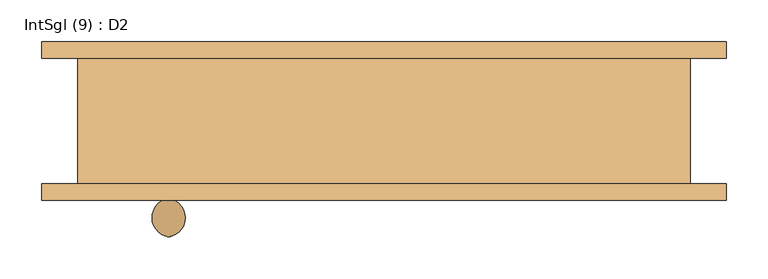
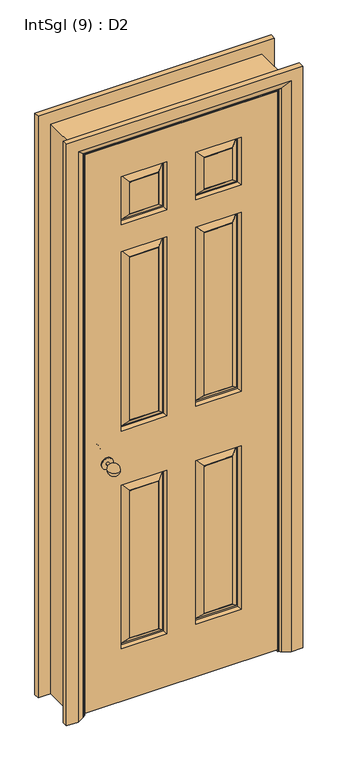
"""IFC4 building model written with IfcOpenShell, lengths in millimetres: door geometry, IntSgl (9) : D2."""

from ifc_helpers import new_model, si_unit, point, frame, origin, place, context, project, spatial, polyline, circle_curve, ellipse_curve, trimmed, outline, extrude, faceted_brep, source, transform, mapped, element, save
from ifc_brep_helpers import plane_surface, cylinder_surface, revolved_surface, advanced_brep


def intsgl_9_d2_a593ccd7(model_context):
    return source(origin(), model_context, "Body", "SolidModel", [
        advanced_brep(
        [(-253.0, -18.0, 900.0), (-263.0, -18.0, 900.0), (-258.0, 26.437411, 900.0), (-253.0, -33.0, 900.0), (-263.0, -33.0, 900.0), (-278.0, -37.0, 900.0), (-238.0, -37.0, 900.0), (-278.0, -33.0, 900.0), (-238.0, -33.0, 900.0)],
        [
            (0, 1, circle_curve(frame((-258.0, -18.0, 900.0), z_axis=(0.0, 1.0, 0.0), x_axis=(-1.0, 0.0, 0.0)), 5.0)),
            (1, 2, circle_curve(frame((-254.8115138, 3.5786495, 900.0), z_axis=(0.0, 0.0, -1.0), x_axis=(0.0, -1.0, 0.0)), 23.0800654)),
            (2, 0, circle_curve(frame((-261.1884862, 3.5786495, 900.0), z_axis=(0.0, 0.0, -1.0), x_axis=(0.0, -1.0, 0.0)), 23.0800654)),
            (1, 0, circle_curve(frame((-258.0, -18.0, 900.0), z_axis=(0.0, 1.0, 0.0), x_axis=(-1.0, 0.0, 0.0)), 5.0)),
            (0, 3),
            (3, 4, circle_curve(frame((-258.0, -33.0, 900.0), z_axis=(0.0, 1.0, 0.0), x_axis=(-1.0, 0.0, 0.0)), 5.0)),
            (4, 1),
            (4, 3, circle_curve(frame((-258.0, -33.0, 900.0), z_axis=(0.0, 1.0, 0.0), x_axis=(-1.0, 0.0, 0.0)), 5.0)),
            (5, 6, circle_curve(frame((-258.0, -37.0, 900.0), z_axis=(0.0, -1.0, 0.0), x_axis=(1.0, 0.0, 0.0)), 20.0)),
            (6, 5, circle_curve(frame((-258.0, -37.0, 900.0), z_axis=(0.0, -1.0, 0.0), x_axis=(1.0, 0.0, 0.0)), 20.0)),
            (7, 8, circle_curve(frame((-258.0, -33.0, 900.0), z_axis=(0.0, 1.0, 0.0), x_axis=(1.0, 0.0, 0.0)), 20.0)),
            (8, 7, circle_curve(frame((-258.0, -33.0, 900.0), z_axis=(0.0, 1.0, 0.0), x_axis=(1.0, 0.0, 0.0)), 20.0)),
            (5, 7),
            (8, 6),
        ],
        [
            revolved_surface(trimmed(ellipse_curve(frame((-254.8115138, 3.5786495, 900.0), z_axis=(0.0, 0.0, 1.0), x_axis=(0.0, -1.0, 0.0)), 23.0800654, 23.0800654), [point((-258.0, 26.437411, 900.0))], [point((-263.0, -18.0, 900.0))], True, "CARTESIAN"), (-258.0, -33.0, 900.0), (0.0, -1.0, 0.0)),
            cylinder_surface(frame((-258.0, -33.0, 900.0), z_axis=(0.0, -1.0, 0.0), x_axis=(-1.0, 0.0, 0.0)), 5.0),
            plane_surface(frame((-238.0, -37.0, 900.0), z_axis=(0.0, -1.0, 0.0), x_axis=(0.0, 0.0, 1.0))),
            plane_surface(frame((-238.0, -33.0, 900.0), z_axis=(0.0, 1.0, 0.0), x_axis=(0.0, 0.0, -1.0))),
            cylinder_surface(frame((-258.0, -33.0, 900.0), z_axis=(0.0, -1.0, 0.0), x_axis=(1.0, 0.0, 0.0)), 20.0),
        ],
        [
            (0, [[1, 2, 3]]),
            (0, [[-2, 4, -3]]),
            (1, [[-1, 5, 6, 7]]),
            (1, [[-4, -7, 8, -5]]),
            (2, [[9, 10]]),
            (3, [[11, 12], [-6, -8]]),
            (4, [[-9, 13, -12, 14]]),
            (4, [[-10, -14, -11, -13]]),
        ],
    ),
        advanced_brep(
        [(-253.0, -94.0, 900.0), (-258.0, -138.437411, 900.0), (-263.0, -94.0, 900.0), (-263.0, -79.0, 900.0), (-253.0, -79.0, 900.0), (-278.0, -75.0, 900.0), (-238.0, -75.0, 900.0), (-278.0, -79.0, 900.0), (-238.0, -79.0, 900.0)],
        [
            (0, 1, circle_curve(frame((-261.1884862, -115.5786495, 900.0), z_axis=(0.0, 0.0, -1.0), x_axis=(0.0, 1.0, 0.0)), 23.0800654)),
            (1, 2, circle_curve(frame((-254.8115138, -115.5786495, 900.0), z_axis=(0.0, 0.0, -1.0), x_axis=(0.0, 1.0, 0.0)), 23.0800654)),
            (2, 0, circle_curve(frame((-258.0, -94.0, 900.0), z_axis=(0.0, -1.0, 0.0), x_axis=(-1.0, 0.0, 0.0)), 5.0)),
            (0, 2, circle_curve(frame((-258.0, -94.0, 900.0), z_axis=(0.0, -1.0, 0.0), x_axis=(-1.0, 0.0, 0.0)), 5.0)),
            (2, 3),
            (3, 4, circle_curve(frame((-258.0, -79.0, 900.0), z_axis=(0.0, -1.0, 0.0), x_axis=(-1.0, 0.0, 0.0)), 5.0)),
            (4, 0),
            (4, 3, circle_curve(frame((-258.0, -79.0, 900.0), z_axis=(0.0, -1.0, 0.0), x_axis=(-1.0, 0.0, 0.0)), 5.0)),
            (5, 6, circle_curve(frame((-258.0, -75.0, 900.0), z_axis=(0.0, 1.0, 0.0), x_axis=(1.0, 0.0, 0.0)), 20.0)),
            (6, 5, circle_curve(frame((-258.0, -75.0, 900.0), z_axis=(0.0, 1.0, 0.0), x_axis=(1.0, 0.0, 0.0)), 20.0)),
            (7, 8, circle_curve(frame((-258.0, -79.0, 900.0), z_axis=(0.0, -1.0, 0.0), x_axis=(1.0, 0.0, 0.0)), 20.0)),
            (8, 7, circle_curve(frame((-258.0, -79.0, 900.0), z_axis=(0.0, -1.0, 0.0), x_axis=(1.0, 0.0, 0.0)), 20.0)),
            (6, 8),
            (7, 5),
        ],
        [
            revolved_surface(trimmed(ellipse_curve(frame((-254.8115138, -115.5786495, 900.0), z_axis=(0.0, 0.0, -1.0), x_axis=(0.0, 1.0, 0.0)), 23.0800654, 23.0800654), [point((-258.0, -138.437411, 900.0))], [point((-263.0, -94.0, 900.0))], True, "CARTESIAN"), (-258.0, -79.0, 900.0), (0.0, 1.0, 0.0)),
            cylinder_surface(frame((-258.0, -79.0, 900.0), z_axis=(0.0, 1.0, 0.0), x_axis=(-1.0, 0.0, 0.0)), 5.0),
            plane_surface(frame((-238.0, -75.0, 900.0), z_axis=(0.0, 1.0, 0.0), x_axis=(0.0, 0.0, 1.0))),
            plane_surface(frame((-238.0, -79.0, 900.0), z_axis=(0.0, -1.0, 0.0), x_axis=(0.0, 0.0, -1.0))),
            cylinder_surface(frame((-258.0, -79.0, 900.0), z_axis=(0.0, 1.0, 0.0), x_axis=(1.0, 0.0, 0.0)), 20.0),
        ],
        [
            (0, [[1, 2, 3]]),
            (0, [[-1, 4, -2]]),
            (1, [[5, 6, 7, -3]]),
            (1, [[-7, 8, -5, -4]]),
            (2, [[9, 10]]),
            (3, [[11, 12], [-8, -6]]),
            (4, [[13, -11, 14, -10]]),
            (4, [[-14, -12, -13, -9]]),
        ],
    ),
        faceted_brep([(-333.0, -37.0, 2058.0), (333.0, -37.0, 2058.0), (333.0, -37.0, 8.0), (-333.0, -37.0, 8.0), (-50.0, -37.0, 800.0), (-208.0, -37.0, 800.0), (-208.0, -37.0, 200.0), (-50.0, -37.0, 200.0), (208.0, -37.0, 800.0), (50.0, -37.0, 800.0), (50.0, -37.0, 200.0), (208.0, -37.0, 200.0), (-50.0, -37.0, 1658.0), (-208.0, -37.0, 1658.0), (-208.0, -37.0, 1000.0), (-50.0, -37.0, 1000.0), (208.0, -37.0, 1658.0), (50.0, -37.0, 1658.0), (50.0, -37.0, 1000.0), (208.0, -37.0, 1000.0), (-50.0, -37.0, 1933.0), (-208.0, -37.0, 1933.0), (-208.0, -37.0, 1758.0), (-50.0, -37.0, 1758.0), (208.0, -37.0, 1933.0), (50.0, -37.0, 1933.0), (50.0, -37.0, 1758.0), (208.0, -37.0, 1758.0), (-80.0, -37.0, 230.0), (-178.0, -37.0, 230.0), (-178.0, -37.0, 770.0), (-80.0, -37.0, 770.0), (178.0, -37.0, 230.0), (80.0, -37.0, 230.0), (80.0, -37.0, 770.0), (178.0, -37.0, 770.0), (-80.0, -37.0, 1030.0), (-178.0, -37.0, 1030.0), (-178.0, -37.0, 1628.0), (-80.0, -37.0, 1628.0), (178.0, -37.0, 1030.0), (80.0, -37.0, 1030.0), (80.0, -37.0, 1628.0), (178.0, -37.0, 1628.0), (-80.0, -37.0, 1788.0), (-178.0, -37.0, 1788.0), (-178.0, -37.0, 1903.0), (-80.0, -37.0, 1903.0), (178.0, -37.0, 1788.0), (80.0, -37.0, 1788.0), (80.0, -37.0, 1903.0), (178.0, -37.0, 1903.0), (-333.0, -75.0, 2058.0), (-333.0, -75.0, 8.0), (333.0, -75.0, 8.0), (333.0, -75.0, 2058.0), (50.0, -75.0, 800.0), (208.0, -75.0, 800.0), (208.0, -75.0, 200.0), (50.0, -75.0, 200.0), (-208.0, -75.0, 800.0), (-50.0, -75.0, 800.0), (-50.0, -75.0, 200.0), (-208.0, -75.0, 200.0), (50.0, -75.0, 1658.0), (208.0, -75.0, 1658.0), (208.0, -75.0, 1000.0), (50.0, -75.0, 1000.0), (-208.0, -75.0, 1658.0), (-50.0, -75.0, 1658.0), (-50.0, -75.0, 1000.0), (-208.0, -75.0, 1000.0), (50.0, -75.0, 1933.0), (208.0, -75.0, 1933.0), (208.0, -75.0, 1758.0), (50.0, -75.0, 1758.0), (-208.0, -75.0, 1933.0), (-50.0, -75.0, 1933.0), (-50.0, -75.0, 1758.0), (-208.0, -75.0, 1758.0), (80.0, -75.0, 230.0), (178.0, -75.0, 230.0), (178.0, -75.0, 770.0), (80.0, -75.0, 770.0), (-178.0, -75.0, 230.0), (-80.0, -75.0, 230.0), (-80.0, -75.0, 770.0), (-178.0, -75.0, 770.0), (80.0, -75.0, 1030.0), (178.0, -75.0, 1030.0), (178.0, -75.0, 1628.0), (80.0, -75.0, 1628.0), (-178.0, -75.0, 1030.0), (-80.0, -75.0, 1030.0), (-80.0, -75.0, 1628.0), (-178.0, -75.0, 1628.0), (80.0, -75.0, 1788.0), (178.0, -75.0, 1788.0), (178.0, -75.0, 1903.0), (80.0, -75.0, 1903.0), (-178.0, -75.0, 1788.0), (-80.0, -75.0, 1788.0), (-80.0, -75.0, 1903.0), (-178.0, -75.0, 1903.0), (80.0, -74.0, 230.0), (80.0, -74.0, 770.0), (58.0, -60.0, 208.0), (78.0, -74.0, 228.0), (78.0, -74.0, 772.0), (58.0, -60.0, 792.0), (53.0, -60.0, 203.0), (53.0, -60.0, 797.0), (178.0, -74.0, 770.0), (180.0, -74.0, 772.0), (200.0, -60.0, 792.0), (205.0, -60.0, 797.0), (178.0, -74.0, 230.0), (180.0, -74.0, 228.0), (200.0, -60.0, 208.0), (205.0, -60.0, 203.0), (-178.0, -74.0, 230.0), (-178.0, -74.0, 770.0), (-200.0, -60.0, 208.0), (-180.0, -74.0, 228.0), (-180.0, -74.0, 772.0), (-200.0, -60.0, 792.0), (-205.0, -60.0, 203.0), (-205.0, -60.0, 797.0), (-80.0, -74.0, 770.0), (-78.0, -74.0, 772.0), (-58.0, -60.0, 792.0), (-53.0, -60.0, 797.0), (-80.0, -74.0, 230.0), (-78.0, -74.0, 228.0), (-58.0, -60.0, 208.0), (-53.0, -60.0, 203.0), (80.0, -74.0, 1030.0), (80.0, -74.0, 1628.0), (58.0, -60.0, 1008.0), (78.0, -74.0, 1028.0), (78.0, -74.0, 1630.0), (58.0, -60.0, 1650.0), (53.0, -60.0, 1003.0), (53.0, -60.0, 1655.0), (178.0, -74.0, 1628.0), (180.0, -74.0, 1630.0), (200.0, -60.0, 1650.0), (205.0, -60.0, 1655.0), (178.0, -74.0, 1030.0), (180.0, -74.0, 1028.0), (200.0, -60.0, 1008.0), (205.0, -60.0, 1003.0), (-178.0, -74.0, 1030.0), (-178.0, -74.0, 1628.0), (-200.0, -60.0, 1008.0), (-180.0, -74.0, 1028.0), (-180.0, -74.0, 1630.0), (-200.0, -60.0, 1650.0), (-205.0, -60.0, 1003.0), (-205.0, -60.0, 1655.0), (-80.0, -74.0, 1628.0), (-78.0, -74.0, 1630.0), (-58.0, -60.0, 1650.0), (-53.0, -60.0, 1655.0), (-80.0, -74.0, 1030.0), (-78.0, -74.0, 1028.0), (-58.0, -60.0, 1008.0), (-53.0, -60.0, 1003.0), (80.0, -74.0, 1788.0), (80.0, -74.0, 1903.0), (58.0, -60.0, 1766.0), (78.0, -74.0, 1786.0), (78.0, -74.0, 1905.0), (58.0, -60.0, 1925.0), (53.0, -60.0, 1761.0), (53.0, -60.0, 1930.0), (178.0, -74.0, 1903.0), (180.0, -74.0, 1905.0), (200.0, -60.0, 1925.0), (205.0, -60.0, 1930.0), (178.0, -74.0, 1788.0), (180.0, -74.0, 1786.0), (200.0, -60.0, 1766.0), (205.0, -60.0, 1761.0), (-178.0, -74.0, 1788.0), (-178.0, -74.0, 1903.0), (-200.0, -60.0, 1766.0), (-180.0, -74.0, 1786.0), (-180.0, -74.0, 1905.0), (-200.0, -60.0, 1925.0), (-205.0, -60.0, 1761.0), (-205.0, -60.0, 1930.0), (-80.0, -74.0, 1903.0), (-78.0, -74.0, 1905.0), (-58.0, -60.0, 1925.0), (-53.0, -60.0, 1930.0), (-80.0, -74.0, 1788.0), (-78.0, -74.0, 1786.0), (-58.0, -60.0, 1766.0), (-53.0, -60.0, 1761.0), (-80.0, -38.0, 230.0), (-80.0, -38.0, 770.0), (-58.0, -52.0, 208.0), (-78.0, -38.0, 228.0), (-78.0, -38.0, 772.0), (-58.0, -52.0, 792.0), (-53.0, -52.0, 203.0), (-53.0, -52.0, 797.0), (-178.0, -38.0, 770.0), (-180.0, -38.0, 772.0), (-200.0, -52.0, 792.0), (-205.0, -52.0, 797.0), (-178.0, -38.0, 230.0), (-180.0, -38.0, 228.0), (-200.0, -52.0, 208.0), (-205.0, -52.0, 203.0), (178.0, -38.0, 230.0), (178.0, -38.0, 770.0), (200.0, -52.0, 208.0), (180.0, -38.0, 228.0), (180.0, -38.0, 772.0), (200.0, -52.0, 792.0), (205.0, -52.0, 203.0), (205.0, -52.0, 797.0), (80.0, -38.0, 770.0), (78.0, -38.0, 772.0), (58.0, -52.0, 792.0), (53.0, -52.0, 797.0), (80.0, -38.0, 230.0), (78.0, -38.0, 228.0), (58.0, -52.0, 208.0), (53.0, -52.0, 203.0), (-80.0, -38.0, 1030.0), (-80.0, -38.0, 1628.0), (-58.0, -52.0, 1008.0), (-78.0, -38.0, 1028.0), (-78.0, -38.0, 1630.0), (-58.0, -52.0, 1650.0), (-53.0, -52.0, 1003.0), (-53.0, -52.0, 1655.0), (-178.0, -38.0, 1628.0), (-180.0, -38.0, 1630.0), (-200.0, -52.0, 1650.0), (-205.0, -52.0, 1655.0), (-178.0, -38.0, 1030.0), (-180.0, -38.0, 1028.0), (-200.0, -52.0, 1008.0), (-205.0, -52.0, 1003.0), (178.0, -38.0, 1030.0), (178.0, -38.0, 1628.0), (200.0, -52.0, 1008.0), (180.0, -38.0, 1028.0), (180.0, -38.0, 1630.0), (200.0, -52.0, 1650.0), (205.0, -52.0, 1003.0), (205.0, -52.0, 1655.0), (80.0, -38.0, 1628.0), (78.0, -38.0, 1630.0), (58.0, -52.0, 1650.0), (53.0, -52.0, 1655.0), (80.0, -38.0, 1030.0), (78.0, -38.0, 1028.0), (58.0, -52.0, 1008.0), (53.0, -52.0, 1003.0), (-80.0, -38.0, 1788.0), (-80.0, -38.0, 1903.0), (-58.0, -52.0, 1766.0), (-78.0, -38.0, 1786.0), (-78.0, -38.0, 1905.0), (-58.0, -52.0, 1925.0), (-53.0, -52.0, 1761.0), (-53.0, -52.0, 1930.0), (-178.0, -38.0, 1903.0), (-180.0, -38.0, 1905.0), (-200.0, -52.0, 1925.0), (-205.0, -52.0, 1930.0), (-178.0, -38.0, 1788.0), (-180.0, -38.0, 1786.0), (-200.0, -52.0, 1766.0), (-205.0, -52.0, 1761.0), (178.0, -38.0, 1788.0), (178.0, -38.0, 1903.0), (200.0, -52.0, 1766.0), (180.0, -38.0, 1786.0), (180.0, -38.0, 1905.0), (200.0, -52.0, 1925.0), (205.0, -52.0, 1761.0), (205.0, -52.0, 1930.0), (80.0, -38.0, 1903.0), (78.0, -38.0, 1905.0), (58.0, -52.0, 1925.0), (53.0, -52.0, 1930.0), (80.0, -38.0, 1788.0), (78.0, -38.0, 1786.0), (58.0, -52.0, 1766.0), (53.0, -52.0, 1761.0)], [[[0, 1, 2, 3], [4, 5, 6, 7], [8, 9, 10, 11], [12, 13, 14, 15], [16, 17, 18, 19], [20, 21, 22, 23], [24, 25, 26, 27]], [[28, 29, 30, 31]], [[32, 33, 34, 35]], [[36, 37, 38, 39]], [[40, 41, 42, 43]], [[44, 45, 46, 47]], [[48, 49, 50, 51]], [[52, 53, 54, 55], [56, 57, 58, 59], [60, 61, 62, 63], [64, 65, 66, 67], [68, 69, 70, 71], [72, 73, 74, 75], [76, 77, 78, 79]], [[80, 81, 82, 83]], [[84, 85, 86, 87]], [[88, 89, 90, 91]], [[92, 93, 94, 95]], [[96, 97, 98, 99]], [[100, 101, 102, 103]], [[3, 53, 52, 0]], [[2, 54, 53, 3]], [[1, 55, 54, 2]], [[0, 52, 55, 1]], [[104, 80, 83, 105]], [[106, 107, 108, 109]], [[56, 59, 110, 111]], [[83, 82, 112, 105]], [[108, 113, 114, 109]], [[111, 115, 57, 56]], [[82, 81, 116, 112]], [[113, 117, 118, 114]], [[115, 119, 58, 57]], [[104, 116, 81, 80]], [[107, 117, 113, 108], [105, 112, 116, 104]], [[106, 118, 117, 107]], [[110, 119, 115, 111], [109, 114, 118, 106]], [[59, 58, 119, 110]], [[120, 84, 87, 121]], [[122, 123, 124, 125]], [[60, 63, 126, 127]], [[87, 86, 128, 121]], [[124, 129, 130, 125]], [[127, 131, 61, 60]], [[86, 85, 132, 128]], [[129, 133, 134, 130]], [[131, 135, 62, 61]], [[120, 132, 85, 84]], [[123, 133, 129, 124], [121, 128, 132, 120]], [[122, 134, 133, 123]], [[126, 135, 131, 127], [125, 130, 134, 122]], [[63, 62, 135, 126]], [[136, 88, 91, 137]], [[138, 139, 140, 141]], [[64, 67, 142, 143]], [[91, 90, 144, 137]], [[140, 145, 146, 141]], [[143, 147, 65, 64]], [[90, 89, 148, 144]], [[145, 149, 150, 146]], [[147, 151, 66, 65]], [[136, 148, 89, 88]], [[139, 149, 145, 140], [137, 144, 148, 136]], [[138, 150, 149, 139]], [[142, 151, 147, 143], [141, 146, 150, 138]], [[67, 66, 151, 142]], [[152, 92, 95, 153]], [[154, 155, 156, 157]], [[68, 71, 158, 159]], [[95, 94, 160, 153]], [[156, 161, 162, 157]], [[159, 163, 69, 68]], [[94, 93, 164, 160]], [[161, 165, 166, 162]], [[163, 167, 70, 69]], [[152, 164, 93, 92]], [[155, 165, 161, 156], [153, 160, 164, 152]], [[154, 166, 165, 155]], [[158, 167, 163, 159], [157, 162, 166, 154]], [[71, 70, 167, 158]], [[168, 96, 99, 169]], [[170, 171, 172, 173]], [[72, 75, 174, 175]], [[99, 98, 176, 169]], [[172, 177, 178, 173]], [[175, 179, 73, 72]], [[98, 97, 180, 176]], [[177, 181, 182, 178]], [[179, 183, 74, 73]], [[168, 180, 97, 96]], [[171, 181, 177, 172], [169, 176, 180, 168]], [[170, 182, 181, 171]], [[174, 183, 179, 175], [173, 178, 182, 170]], [[75, 74, 183, 174]], [[184, 100, 103, 185]], [[186, 187, 188, 189]], [[76, 79, 190, 191]], [[103, 102, 192, 185]], [[188, 193, 194, 189]], [[191, 195, 77, 76]], [[102, 101, 196, 192]], [[193, 197, 198, 194]], [[195, 199, 78, 77]], [[184, 196, 101, 100]], [[187, 197, 193, 188], [185, 192, 196, 184]], [[186, 198, 197, 187]], [[190, 199, 195, 191], [189, 194, 198, 186]], [[79, 78, 199, 190]], [[200, 28, 31, 201]], [[202, 203, 204, 205]], [[4, 7, 206, 207]], [[31, 30, 208, 201]], [[204, 209, 210, 205]], [[207, 211, 5, 4]], [[30, 29, 212, 208]], [[209, 213, 214, 210]], [[211, 215, 6, 5]], [[200, 212, 29, 28]], [[203, 213, 209, 204], [201, 208, 212, 200]], [[202, 214, 213, 203]], [[206, 215, 211, 207], [205, 210, 214, 202]], [[7, 6, 215, 206]], [[216, 32, 35, 217]], [[218, 219, 220, 221]], [[8, 11, 222, 223]], [[35, 34, 224, 217]], [[220, 225, 226, 221]], [[223, 227, 9, 8]], [[34, 33, 228, 224]], [[225, 229, 230, 226]], [[227, 231, 10, 9]], [[216, 228, 33, 32]], [[219, 229, 225, 220], [217, 224, 228, 216]], [[218, 230, 229, 219]], [[222, 231, 227, 223], [221, 226, 230, 218]], [[11, 10, 231, 222]], [[232, 36, 39, 233]], [[234, 235, 236, 237]], [[12, 15, 238, 239]], [[39, 38, 240, 233]], [[236, 241, 242, 237]], [[239, 243, 13, 12]], [[38, 37, 244, 240]], [[241, 245, 246, 242]], [[243, 247, 14, 13]], [[232, 244, 37, 36]], [[235, 245, 241, 236], [233, 240, 244, 232]], [[234, 246, 245, 235]], [[238, 247, 243, 239], [237, 242, 246, 234]], [[15, 14, 247, 238]], [[248, 40, 43, 249]], [[250, 251, 252, 253]], [[16, 19, 254, 255]], [[43, 42, 256, 249]], [[252, 257, 258, 253]], [[255, 259, 17, 16]], [[42, 41, 260, 256]], [[257, 261, 262, 258]], [[259, 263, 18, 17]], [[248, 260, 41, 40]], [[251, 261, 257, 252], [249, 256, 260, 248]], [[250, 262, 261, 251]], [[254, 263, 259, 255], [253, 258, 262, 250]], [[19, 18, 263, 254]], [[264, 44, 47, 265]], [[266, 267, 268, 269]], [[20, 23, 270, 271]], [[47, 46, 272, 265]], [[268, 273, 274, 269]], [[271, 275, 21, 20]], [[46, 45, 276, 272]], [[273, 277, 278, 274]], [[275, 279, 22, 21]], [[264, 276, 45, 44]], [[267, 277, 273, 268], [265, 272, 276, 264]], [[266, 278, 277, 267]], [[270, 279, 275, 271], [269, 274, 278, 266]], [[23, 22, 279, 270]], [[280, 48, 51, 281]], [[282, 283, 284, 285]], [[24, 27, 286, 287]], [[51, 50, 288, 281]], [[284, 289, 290, 285]], [[287, 291, 25, 24]], [[50, 49, 292, 288]], [[289, 293, 294, 290]], [[291, 295, 26, 25]], [[280, 292, 49, 48]], [[283, 293, 289, 284], [281, 288, 292, 280]], [[282, 294, 293, 283]], [[286, 295, 291, 287], [285, 290, 294, 282]], [[27, 26, 295, 286]]]),
        faceted_brep([(-335.0, -75.0, 0.0), (-367.0, -75.0, 0.0), (-367.0, 75.0, 0.0), (-335.0, 75.0, 0.0), (-335.0, 75.0, 2060.0), (-335.0, -75.0, 2060.0), (-367.0, 75.0, 2092.0), (-367.0, -75.0, 2092.0), (335.0, -75.0, 0.0), (335.0, 75.0, 0.0), (367.0, 75.0, 0.0), (367.0, -75.0, 0.0), (335.0, -75.0, 2060.0), (367.0, -75.0, 2092.0), (367.0, 75.0, 2092.0), (335.0, 75.0, 2060.0)], [[[0, 1, 2, 3]], [[3, 4, 5, 0]], [[2, 6, 4, 3]], [[1, 7, 6, 2]], [[0, 5, 7, 1]], [[8, 9, 10, 11]], [[12, 8, 11, 13]], [[13, 11, 10, 14]], [[14, 10, 9, 15]], [[15, 9, 8, 12]], [[4, 15, 12, 5]], [[6, 14, 15, 4]], [[7, 13, 14, 6]], [[5, 12, 13, 7]]]),
        extrude(outline(polyline([(0.0, -316.0), (2041.0, -316.0), (2041.0, 316.0), (0.0, 316.0), (0.0, 335.0), (2060.0, 335.0), (2060.0, -335.0), (0.0, -335.0), (0.0, -316.0)])), frame((0.0, -35.0, 0.0), z_axis=(0.0, 1.0, 0.0), x_axis=(0.0, 0.0, 1.0)), (0.0, 0.0, 1.0), 32.0),
        advanced_brep(
        [(-410.0, 95.0, 0.0), (-370.0, 95.0, 0.0), (-344.0, 81.0, 0.0), (-340.0, 75.0, 0.0), (-410.0, 75.0, 0.0), (-410.0, 75.0, 2135.0), (-410.0, 95.0, 2135.0), (-340.0, 75.0, 2065.0), (340.0, 75.0, 2065.0), (340.0, 75.0, 0.0), (410.0, 75.0, 0.0), (410.0, 75.0, 2135.0), (-344.0, 81.0, 2069.0), (-370.0, 95.0, 2095.0), (410.0, 95.0, 2135.0), (410.0, 95.0, 0.0), (370.0, 95.0, 0.0), (370.0, 95.0, 2095.0), (344.0, 81.0, 0.0), (344.0, 81.0, 2069.0)],
        [
            (0, 1),
            (1, 2),
            (2, 3, circle_curve(frame((-348.0, 74.0, 0.0), z_axis=(0.0, 0.0, -1.0), x_axis=(-1.0, 0.0, 0.0)), 8.0622577)),
            (3, 4),
            (4, 0),
            (4, 5),
            (5, 6),
            (6, 0),
            (3, 7),
            (7, 8),
            (8, 9),
            (9, 10),
            (10, 11),
            (11, 5),
            (2, 12),
            (12, 7, ellipse_curve(frame((-348.0, 74.0, 2073.0), z_axis=(-0.7071067811865475, 0.0, -0.7071067811865475), x_axis=(0.7071067811865474, 0.0, -0.7071067811865476)), 11.4017543, 8.0622577)),
            (1, 13),
            (13, 12),
            (6, 14),
            (14, 15),
            (15, 16),
            (16, 17),
            (17, 13),
            (10, 15),
            (14, 11),
            (9, 18, circle_curve(frame((348.0, 74.0, 0.0), z_axis=(0.0, 0.0, -1.0), x_axis=(1.0, 0.0, 0.0)), 8.0622577)),
            (18, 16),
            (19, 18),
            (8, 19, ellipse_curve(frame((348.0, 74.0, 2073.0), z_axis=(0.7071067811865475, 0.0, -0.7071067811865475), x_axis=(0.7071067811865474, 0.0, 0.7071067811865476)), 11.4017543, 8.0622577)),
            (19, 17),
            (12, 19),
        ],
        [
            plane_surface(frame((-340.0, 75.0, 0.0), z_axis=(0.0, 0.0, -1.0), x_axis=(0.0, 1.0, 0.0))),
            plane_surface(frame((-410.0, 95.0, 0.0), z_axis=(-1.0, 0.0, 0.0), x_axis=(0.0, 0.0, 1.0))),
            plane_surface(frame((-410.0, 75.0, 0.0), z_axis=(0.0, -1.0, 0.0), x_axis=(0.0, 0.0, 1.0))),
            cylinder_surface(frame((-348.0, 74.0, 0.0), z_axis=(0.0, 0.0, -1.0), x_axis=(-1.0, 0.0, 0.0)), 8.0622577),
            plane_surface(frame((-344.0, 81.0, 0.0), z_axis=(0.4740998230350183, 0.8804710999221749, 0.0), x_axis=(0.0, 0.0, 1.0))),
            plane_surface(frame((-370.0, 95.0, 0.0), z_axis=(0.0, 1.0, 0.0), x_axis=(0.0, 0.0, 1.0))),
            plane_surface(frame((410.0, 95.0, 2135.0), z_axis=(1.0, 0.0, 0.0), x_axis=(0.0, 0.0, -1.0))),
            plane_surface(frame((340.0, 75.0, 0.0), z_axis=(0.0, 0.0, -1.0), x_axis=(0.0, 1.0, 0.0))),
            cylinder_surface(frame((348.0, 74.0, 2065.0), z_axis=(0.0, 0.0, 1.0), x_axis=(1.0, 0.0, 0.0)), 8.0622577),
            plane_surface(frame((344.0, 81.0, 2069.0), z_axis=(-0.4740998230350183, 0.8804710999221749, 0.0), x_axis=(0.0, 0.0, -1.0))),
            plane_surface(frame((-410.0, 95.0, 2135.0), z_axis=(0.0, 0.0, 1.0), x_axis=(1.0, 0.0, 0.0))),
            cylinder_surface(frame((-340.0, 74.0, 2073.0), z_axis=(-1.0, 0.0, 0.0), x_axis=(0.0, 0.0, 1.0)), 8.0622577),
            plane_surface(frame((-344.0, 81.0, 2069.0), z_axis=(0.0, 0.8804710999221749, -0.4740998230350183), x_axis=(1.0, 0.0, 0.0))),
        ],
        [
            (0, [[1, 2, 3, 4, 5]]),
            (1, [[6, 7, 8, -5]]),
            (2, [[9, 10, 11, 12, 13, 14, -6, -4]]),
            (3, [[15, 16, -9, -3]]),
            (4, [[17, 18, -15, -2]]),
            (5, [[-8, 19, 20, 21, 22, 23, -17, -1]]),
            (6, [[-13, 24, -20, 25]]),
            (7, [[-24, -12, 26, 27, -21]]),
            (8, [[28, -26, -11, 29]]),
            (9, [[-22, -27, -28, 30]]),
            (10, [[-14, -25, -19, -7]]),
            (11, [[31, -29, -10, -16]]),
            (12, [[-23, -30, -31, -18]]),
        ],
    ),
        advanced_brep(
        [(410.0, -95.0, 0.0), (370.0, -95.0, 0.0), (344.0, -81.0, 0.0), (340.0, -75.0, 0.0), (410.0, -75.0, 0.0), (410.0, -75.0, 2135.0), (410.0, -95.0, 2135.0), (340.0, -75.0, 2065.0), (-340.0, -75.0, 2065.0), (-340.0, -75.0, 0.0), (-410.0, -75.0, 0.0), (-410.0, -75.0, 2135.0), (344.0, -81.0, 2069.0), (370.0, -95.0, 2095.0), (-410.0, -95.0, 2135.0), (-410.0, -95.0, 0.0), (-370.0, -95.0, 0.0), (-370.0, -95.0, 2095.0), (-344.0, -81.0, 0.0), (-344.0, -81.0, 2069.0)],
        [
            (0, 1),
            (1, 2),
            (2, 3, circle_curve(frame((348.0, -74.0, 0.0), z_axis=(0.0, 0.0, -1.0), x_axis=(1.0, 0.0, 0.0)), 8.0622577)),
            (3, 4),
            (4, 0),
            (4, 5),
            (5, 6),
            (6, 0),
            (3, 7),
            (7, 8),
            (8, 9),
            (9, 10),
            (10, 11),
            (11, 5),
            (2, 12),
            (12, 7, ellipse_curve(frame((348.0, -74.0, 2073.0), z_axis=(0.7071067811865475, 0.0, -0.7071067811865475), x_axis=(-0.7071067811865474, 0.0, -0.7071067811865476)), 11.4017543, 8.0622577)),
            (1, 13),
            (13, 12),
            (6, 14),
            (14, 15),
            (15, 16),
            (16, 17),
            (17, 13),
            (10, 15),
            (14, 11),
            (9, 18, circle_curve(frame((-348.0, -74.0, 0.0), z_axis=(0.0, 0.0, -1.0), x_axis=(-1.0, 0.0, 0.0)), 8.0622577)),
            (18, 16),
            (19, 18),
            (8, 19, ellipse_curve(frame((-348.0, -74.0, 2073.0), z_axis=(-0.7071067811865475, 0.0, -0.7071067811865475), x_axis=(-0.7071067811865474, 0.0, 0.7071067811865476)), 11.4017543, 8.0622577)),
            (19, 17),
            (12, 19),
        ],
        [
            plane_surface(frame((340.0, -75.0, 0.0), z_axis=(0.0, 0.0, -1.0), x_axis=(0.0, -1.0, 0.0))),
            plane_surface(frame((410.0, -95.0, 0.0), z_axis=(1.0, 0.0, 0.0), x_axis=(0.0, 0.0, 1.0))),
            plane_surface(frame((410.0, -75.0, 0.0), z_axis=(0.0, 1.0, 0.0), x_axis=(0.0, 0.0, 1.0))),
            cylinder_surface(frame((348.0, -74.0, 0.0), z_axis=(0.0, 0.0, -1.0), x_axis=(1.0, 0.0, 0.0)), 8.0622577),
            plane_surface(frame((344.0, -81.0, 0.0), z_axis=(-0.4740998230350183, -0.8804710999221749, 0.0), x_axis=(0.0, 0.0, 1.0))),
            plane_surface(frame((370.0, -95.0, 0.0), z_axis=(0.0, -1.0, 0.0), x_axis=(0.0, 0.0, 1.0))),
            plane_surface(frame((-410.0, -95.0, 2135.0), z_axis=(-1.0, 0.0, 0.0), x_axis=(0.0, 0.0, -1.0))),
            plane_surface(frame((-340.0, -75.0, 0.0), z_axis=(0.0, 0.0, -1.0), x_axis=(0.0, -1.0, 0.0))),
            cylinder_surface(frame((-348.0, -74.0, 2065.0), z_axis=(0.0, 0.0, 1.0), x_axis=(-1.0, 0.0, 0.0)), 8.0622577),
            plane_surface(frame((-344.0, -81.0, 2069.0), z_axis=(0.4740998230350183, -0.8804710999221749, 0.0), x_axis=(0.0, 0.0, -1.0))),
            plane_surface(frame((410.0, -95.0, 2135.0), z_axis=(0.0, 0.0, 1.0), x_axis=(-1.0, 0.0, 0.0))),
            cylinder_surface(frame((340.0, -74.0, 2073.0), z_axis=(1.0, 0.0, 0.0), x_axis=(0.0, 0.0, 1.0)), 8.0622577),
            plane_surface(frame((344.0, -81.0, 2069.0), z_axis=(0.0, -0.8804710999221749, -0.4740998230350183), x_axis=(-1.0, 0.0, 0.0))),
        ],
        [
            (0, [[1, 2, 3, 4, 5]]),
            (1, [[6, 7, 8, -5]]),
            (2, [[9, 10, 11, 12, 13, 14, -6, -4]]),
            (3, [[15, 16, -9, -3]]),
            (4, [[17, 18, -15, -2]]),
            (5, [[-8, 19, 20, 21, 22, 23, -17, -1]]),
            (6, [[-13, 24, -20, 25]]),
            (7, [[-24, -12, 26, 27, -21]]),
            (8, [[28, -26, -11, 29]]),
            (9, [[-22, -27, -28, 30]]),
            (10, [[-14, -25, -19, -7]]),
            (11, [[31, -29, -10, -16]]),
            (12, [[-23, -30, -31, -18]]),
        ],
    ),
    ])


if __name__ == "__main__":
    model = new_model("IFC4")
    model_context = context("Model", 3, world=origin())
    ifc_project = project(units=[si_unit("LENGTHUNIT", "METRE", prefix="MILLI")], contexts=[model_context])
    site = spatial("IfcSite", under=ifc_project)
    building = spatial("IfcBuilding", under=site)
    placement = place(None, origin())
    intsgl_9_d2_shape = intsgl_9_d2_a593ccd7(model_context)
    element("IfcDoor", 1, ObjectType="IntSgl (9) : D2", at=placement, inside=building, context=model_context, shape_type="MappedRepresentation", body=[
        mapped(intsgl_9_d2_shape, transform((0.0, 0.0, 0.0), x_axis=(1.0, 0.0, 0.0), y_axis=(0.0, 1.0, 0.0), z_axis=(0.0, 0.0, 1.0))),
    ])
    save(model, "model.ifc")

# Revit data of these elements
# Type "IntSgl (9) : D2"
#   Type Mark = "50"
#   Operation = "SingleSwingRight"
#   Manufacturer = "Revit"
#   Keynote = "L20"
#   UnderCut = 8 mm
#   Tolerance = 2 mm
#   Thickness = 38 mm
#   Structural Tolerance = 8 mm
#   StopDepth = 32 mm
#   Stop Thickness = 19 mm
#   Stile Top Rail = 125 mm
#   Stile Shutting = 125 mm
#   Stile Muntin Rail = 100 mm
#   Stile Lock Rail = 200 mm
#   Stile Intermediate/Frieze = 100 mm
#   Stile Hanging = 125 mm
#   Stile Bottom Rail = 200 mm
#   Rough Width = 750 mm
#   Rough Height = 2100 mm
#   Height to Top Lock Rail = 1000 mm
#   Handle Z Distance = 900 mm
#   Handle X Distance = 75 mm
#   Frame Thickness = 32 mm
#   Door Panel Width = 666 mm
#   Height = 2100 mm
#   Width = 750 mm
#   Door Panel Thickness = 38 mm
#   Door Panel Offset = 0 mm
#   Door Panel Height = 2050 mm
#   Architrave Setback = 5 mm
#   Vis - Ironmongery = yes
#   Material Ironmongery = Door - Handle
#   Material Frame = Door - Frame/Mullion
#   Material Door = Door - Panel
#   Material Architrave = Door - Architrave
#   Function = (empty or 0)
#   Wall Closure = (empty or 0)
# Element 1 (IfcDoor, "IntSgl (9) : D2")
#   Materials on its faces: "Door - Panel", "Door - Architrave", "Door - Frame/Mullion", "Door - Handle"
# Materials
#   "Door - Handle": colour RGB 247 247 247, transparency 0
#   "Door - Frame/Mullion": colour RGB 212 179 113, transparency 0
#   "Door - Panel": colour RGB 154 90 5, transparency 0
#   "Door - Architrave": colour RGB 154 90 5, transparency 0
